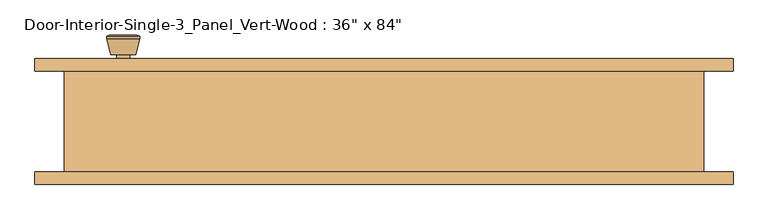
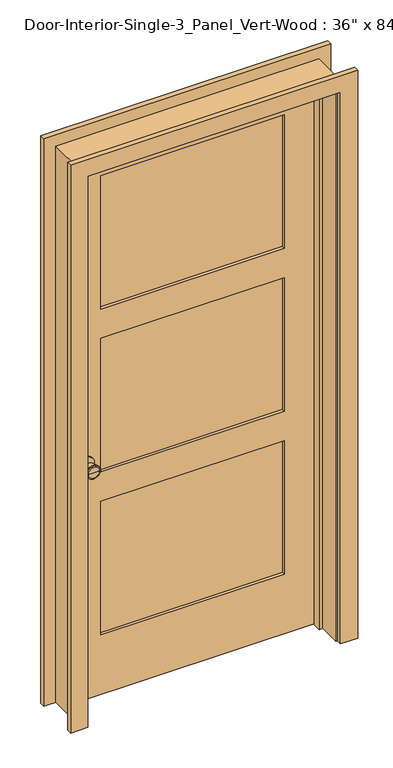
"""IFC4 building model written with IfcOpenShell, lengths in millimetres: door geometry."""

from ifc_helpers import new_model, si_unit, point, frame, frame_2d, origin, place, context, project, spatial, polyline, circle_curve, trimmed, segment, composite_curve, outline, extrude, faceted_brep, source, transform, mapped, element, save
from ifc_brep_helpers import plane_surface, cylinder_surface, revolved_surface, advanced_brep


def door_8959c651(model_context):
    return source(origin(), model_context, "Body", "SolidModel", [
        advanced_brep(
        [(-393.7, 32.1, 914.4), (-383.7, 32.1, 914.4), (-403.7, 32.1, 914.4), (-373.2241324, -16.9, 914.4), (-393.7, -16.9, 914.4), (-414.1758676, -16.9, 914.4), (-368.7, -15.0721319, 914.4), (-418.7, -15.0721319, 914.4), (-368.7, -11.6084537, 914.4), (-418.7, -11.6084537, 914.4), (-375.063764, 13.1, 914.4), (-412.336236, 13.1, 914.4), (-383.7, 13.1, 914.4), (-403.7, 13.1, 914.4)],
        [
            (0, 1),
            (1, 2, circle_curve(frame((-393.7, 32.1, 914.4), z_axis=(0.0, 1.0, 0.0), x_axis=(-1.0, 0.0, 0.0)), 10.0)),
            (2, 0),
            (2, 1, circle_curve(frame((-393.7, 32.1, 914.4), z_axis=(0.0, 1.0, 0.0), x_axis=(-1.0, 0.0, 0.0)), 10.0)),
            (3, 4),
            (4, 5),
            (5, 3, circle_curve(frame((-393.7, -16.9, 914.4), z_axis=(0.0, -1.0, 0.0), x_axis=(-1.0, 0.0, 0.0)), 20.4758676)),
            (3, 5, circle_curve(frame((-393.7, -16.9, 914.4), z_axis=(0.0, -1.0, 0.0), x_axis=(-1.0, 0.0, 0.0)), 20.4758676)),
            (6, 3),
            (5, 7),
            (7, 6, circle_curve(frame((-393.7, -15.0721319, 914.4), z_axis=(0.0, -1.0, 0.0), x_axis=(-1.0, 0.0, 0.0)), 25.0)),
            (6, 7, circle_curve(frame((-393.7, -15.0721319, 914.4), z_axis=(0.0, -1.0, 0.0), x_axis=(-1.0, 0.0, 0.0)), 25.0)),
            (8, 6),
            (7, 9),
            (9, 8, circle_curve(frame((-393.7, -11.6084537, 914.4), z_axis=(0.0, -1.0, 0.0), x_axis=(-1.0, 0.0, 0.0)), 25.0)),
            (8, 9, circle_curve(frame((-393.7, -11.6084537, 914.4), z_axis=(0.0, -1.0, 0.0), x_axis=(-1.0, 0.0, 0.0)), 25.0)),
            (10, 8),
            (9, 11),
            (11, 10, circle_curve(frame((-393.7, 13.1, 914.4), z_axis=(0.0, -1.0, 0.0), x_axis=(-1.0, 0.0, 0.0)), 18.636236)),
            (10, 11, circle_curve(frame((-393.7, 13.1, 914.4), z_axis=(0.0, -1.0, 0.0), x_axis=(-1.0, 0.0, 0.0)), 18.636236)),
            (12, 10),
            (11, 13),
            (13, 12, circle_curve(frame((-393.7, 13.1, 914.4), z_axis=(0.0, -1.0, 0.0), x_axis=(-1.0, 0.0, 0.0)), 10.0)),
            (12, 13, circle_curve(frame((-393.7, 13.1, 914.4), z_axis=(0.0, -1.0, 0.0), x_axis=(-1.0, 0.0, 0.0)), 10.0)),
            (1, 12),
            (13, 2),
        ],
        [
            plane_surface(frame((-393.7, 32.1, 914.4), z_axis=(0.0, 1.0, 0.0), x_axis=(-1.0, 0.0, 0.0))),
            plane_surface(frame((-393.7, -16.9, 914.4), z_axis=(0.0, -1.0, 0.0), x_axis=(-1.0, 0.0, 0.0))),
            revolved_surface(polyline([(-414.1758676, -16.9, 914.4), (-418.7, -15.0721319, 914.4)]), (-393.7, 32.1, 914.4), (0.0, 1.0, 0.0)),
            cylinder_surface(frame((-393.7, 32.1, 914.4), z_axis=(0.0, 1.0, 0.0), x_axis=(-1.0, 0.0, 0.0)), 25.0),
            revolved_surface(polyline([(-418.7, -11.6084537, 914.4), (-412.336236, 13.1, 914.4)]), (-393.7, 32.1, 914.4), (0.0, 1.0, 0.0)),
            plane_surface(frame((-393.7, 13.1, 914.4), z_axis=(0.0, 1.0, 0.0), x_axis=(-1.0, 0.0, 0.0))),
            cylinder_surface(frame((-393.7, 32.1, 914.4), z_axis=(0.0, 1.0, 0.0), x_axis=(-1.0, 0.0, 0.0)), 10.0),
        ],
        [
            (0, [[1, 2, 3]]),
            (0, [[-3, 4, -1]]),
            (1, [[5, 6, 7]]),
            (1, [[-6, -5, 8]]),
            (2, [[9, -7, 10, 11]]),
            (2, [[-10, -8, -9, 12]]),
            (3, [[13, -11, 14, 15]]),
            (3, [[-14, -12, -13, 16]]),
            (4, [[17, -15, 18, 19]]),
            (4, [[-18, -16, -17, 20]]),
            (5, [[21, -19, 22, 23]]),
            (5, [[-22, -20, -21, 24]]),
            (6, [[25, -23, 26, -2]]),
            (6, [[-26, -24, -25, -4]]),
        ],
    ),
        extrude(outline(composite_curve([segment(trimmed(circle_curve(frame_2d((914.4, -393.7)), 30.0), [point((914.4, -423.7))], [point((914.4, -363.7))], False, "CARTESIAN"), True, "CONTINUOUS"), segment(trimmed(circle_curve(frame_2d((914.4, -393.7)), 30.0), [point((914.4, -363.7))], [point((914.4, -423.7))], False, "CARTESIAN"), True, "CONTINUOUS")], self_intersect=False)), frame((0.0, 32.1, 0.0), z_axis=(0.0, 1.0, 0.0), x_axis=(0.0, 0.0, 1.0)), (0.0, 0.0, 1.0), 6.0),
        advanced_brep(
        [(-393.7, 79.025, 914.4), (-403.7, 79.025, 914.4), (-383.7, 79.025, 914.4), (-373.2241324, 128.025, 914.4), (-414.1758676, 128.025, 914.4), (-393.7, 128.025, 914.4), (-368.7, 126.1971319, 914.4), (-418.7, 126.1971319, 914.4), (-368.7, 122.7334537, 914.4), (-418.7, 122.7334537, 914.4), (-375.063764, 98.025, 914.4), (-412.336236, 98.025, 914.4), (-383.7, 98.025, 914.4), (-403.7, 98.025, 914.4)],
        [
            (0, 1),
            (1, 2, circle_curve(frame((-393.7, 79.025, 914.4), z_axis=(0.0, -1.0, 0.0), x_axis=(-1.0, 0.0, 0.0)), 10.0)),
            (2, 0),
            (2, 1, circle_curve(frame((-393.7, 79.025, 914.4), z_axis=(0.0, -1.0, 0.0), x_axis=(-1.0, 0.0, 0.0)), 10.0)),
            (3, 4, circle_curve(frame((-393.7, 128.025, 914.4), z_axis=(0.0, 1.0, 0.0), x_axis=(-1.0, 0.0, 0.0)), 20.4758676)),
            (4, 5),
            (5, 3),
            (4, 3, circle_curve(frame((-393.7, 128.025, 914.4), z_axis=(0.0, 1.0, 0.0), x_axis=(-1.0, 0.0, 0.0)), 20.4758676)),
            (6, 7, circle_curve(frame((-393.7, 126.1971319, 914.4), z_axis=(0.0, 1.0, 0.0), x_axis=(-1.0, 0.0, 0.0)), 25.0)),
            (7, 4),
            (3, 6),
            (7, 6, circle_curve(frame((-393.7, 126.1971319, 914.4), z_axis=(0.0, 1.0, 0.0), x_axis=(-1.0, 0.0, 0.0)), 25.0)),
            (8, 9, circle_curve(frame((-393.7, 122.7334537, 914.4), z_axis=(0.0, 1.0, 0.0), x_axis=(-1.0, 0.0, 0.0)), 25.0)),
            (9, 7),
            (6, 8),
            (9, 8, circle_curve(frame((-393.7, 122.7334537, 914.4), z_axis=(0.0, 1.0, 0.0), x_axis=(-1.0, 0.0, 0.0)), 25.0)),
            (10, 11, circle_curve(frame((-393.7, 98.025, 914.4), z_axis=(0.0, 1.0, 0.0), x_axis=(-1.0, 0.0, 0.0)), 18.636236)),
            (11, 9),
            (8, 10),
            (11, 10, circle_curve(frame((-393.7, 98.025, 914.4), z_axis=(0.0, 1.0, 0.0), x_axis=(-1.0, 0.0, 0.0)), 18.636236)),
            (12, 13, circle_curve(frame((-393.7, 98.025, 914.4), z_axis=(0.0, 1.0, 0.0), x_axis=(-1.0, 0.0, 0.0)), 10.0)),
            (13, 11),
            (10, 12),
            (13, 12, circle_curve(frame((-393.7, 98.025, 914.4), z_axis=(0.0, 1.0, 0.0), x_axis=(-1.0, 0.0, 0.0)), 10.0)),
            (1, 13),
            (12, 2),
        ],
        [
            plane_surface(frame((-393.7, 79.025, 914.4), z_axis=(0.0, -1.0, 0.0), x_axis=(-1.0, 0.0, 0.0))),
            plane_surface(frame((-393.7, 128.025, 914.4), z_axis=(0.0, 1.0, 0.0), x_axis=(-1.0, 0.0, 0.0))),
            revolved_surface(polyline([(-414.1758676, 128.025, 914.4), (-418.7, 126.1971319, 914.4)]), (-393.7, 79.025, 914.4), (0.0, -1.0, 0.0)),
            cylinder_surface(frame((-393.7, 79.025, 914.4), z_axis=(0.0, -1.0, 0.0), x_axis=(-1.0, 0.0, 0.0)), 25.0),
            revolved_surface(polyline([(-418.7, 122.7334537, 914.4), (-412.336236, 98.025, 914.4)]), (-393.7, 79.025, 914.4), (0.0, -1.0, 0.0)),
            plane_surface(frame((-393.7, 98.025, 914.4), z_axis=(0.0, -1.0, 0.0), x_axis=(-1.0, 0.0, 0.0))),
            cylinder_surface(frame((-393.7, 79.025, 914.4), z_axis=(0.0, -1.0, 0.0), x_axis=(-1.0, 0.0, 0.0)), 10.0),
        ],
        [
            (0, [[1, 2, 3]]),
            (0, [[-3, 4, -1]]),
            (1, [[5, 6, 7]]),
            (1, [[8, -7, -6]]),
            (2, [[9, 10, -5, 11]]),
            (2, [[12, -11, -8, -10]]),
            (3, [[13, 14, -9, 15]]),
            (3, [[16, -15, -12, -14]]),
            (4, [[17, 18, -13, 19]]),
            (4, [[20, -19, -16, -18]]),
            (5, [[21, 22, -17, 23]]),
            (5, [[24, -23, -20, -22]]),
            (6, [[-2, 25, -21, 26]]),
            (6, [[-4, -26, -24, -25]]),
        ],
    ),
        extrude(outline(composite_curve([segment(trimmed(circle_curve(frame_2d((914.4, -393.7)), 30.0), [point((914.4, -423.7))], [point((914.4, -363.7))], False, "CARTESIAN"), True, "CONTINUOUS"), segment(trimmed(circle_curve(frame_2d((914.4, -393.7)), 30.0), [point((914.4, -363.7))], [point((914.4, -423.7))], False, "CARTESIAN"), True, "CONTINUOUS")], self_intersect=False)), frame((0.0, 73.025, 0.0), z_axis=(0.0, 1.0, 0.0), x_axis=(0.0, 0.0, 1.0)), (0.0, 0.0, 1.0), 6.0),
        extrude(outline(polyline([(336.55, 49.7416667), (-336.55, 49.7416667), (-336.55, 61.3833333), (336.55, 61.3833333), (336.55, 49.7416667)])), frame((0.0, 0.0, 1496.4833333), z_axis=(0.0, 0.0, 1.0), x_axis=(1.0, 0.0, 0.0)), (0.0, 0.0, 1.0), 518.0541667),
        extrude(outline(polyline([(336.55, 49.7416667), (-336.55, 49.7416667), (-336.55, 61.3833333), (336.55, 61.3833333), (336.55, 49.7416667)])), frame((0.0, 0.0, 231.775), z_axis=(0.0, 0.0, 1.0), x_axis=(1.0, 0.0, 0.0)), (0.0, 0.0, 1.0), 518.0541667),
        extrude(outline(polyline([(336.55, 49.7416667), (-336.55, 49.7416667), (-336.55, 61.3833333), (336.55, 61.3833333), (336.55, 49.7416667)])), frame((0.0, 0.0, 864.1291667), z_axis=(0.0, 0.0, 1.0), x_axis=(1.0, 0.0, 0.0)), (0.0, 0.0, 1.0), 518.0541667),
        extrude(outline(polyline([(2133.6, -457.2), (0.0, -457.2), (0.0, 457.2), (2133.6, 457.2), (2133.6, -457.2)]), holes=[polyline([(2014.5375, -336.55), (2014.5375, 336.55), (1496.4833333, 336.55), (1496.4833333, -336.55), (2014.5375, -336.55)]), polyline([(749.8291667, -336.55), (749.8291667, 336.55), (231.775, 336.55), (231.775, -336.55), (749.8291667, -336.55)]), polyline([(1382.1833333, -336.55), (1382.1833333, 336.55), (864.1291667, 336.55), (864.1291667, -336.55), (1382.1833333, -336.55)])]), frame((0.0, 38.1, 0.0), z_axis=(0.0, 1.0, 0.0), x_axis=(0.0, 0.0, 1.0)), (0.0, 0.0, 1.0), 34.925),
        faceted_brep([(482.6, 73.025, 0.0), (482.6, -79.375, 0.0), (457.2, -79.375, 0.0), (457.2, 3.175, 0.0), (444.5, 3.175, 0.0), (444.5, 38.1, 0.0), (457.2, 38.1, 0.0), (457.2, 73.025, 0.0), (482.6, 73.025, 2159.0), (482.6, -79.375, 2159.0), (-482.6, -79.375, 2159.0), (-482.6, -79.375, 0.0), (-457.2, -79.375, 0.0), (-457.2, -79.375, 2133.6), (457.2, -79.375, 2133.6), (457.2, 3.175, 2133.6), (-457.2, 3.175, 2133.6), (-457.2, 3.175, 0.0), (-444.5, 3.175, 0.0), (-444.5, 3.175, 2120.9), (444.5, 3.175, 2120.9), (444.5, 38.1, 2120.9), (-444.5, 38.1, 2120.9), (-444.5, 38.1, 0.0), (-457.2, 38.1, 0.0), (-457.2, 38.1, 2133.6), (457.2, 38.1, 2133.6), (457.2, 73.025, 2133.6), (-457.2, 73.025, 2133.6), (-457.2, 73.025, 0.0), (-482.6, 73.025, 0.0), (-482.6, 73.025, 2159.0)], [[[0, 1, 2, 3, 4, 5, 6, 7]], [[1, 0, 8, 9]], [[2, 1, 9, 10, 11, 12, 13, 14]], [[3, 2, 14, 15]], [[4, 3, 15, 16, 17, 18, 19, 20]], [[5, 4, 20, 21]], [[6, 5, 21, 22, 23, 24, 25, 26]], [[7, 6, 26, 27]], [[0, 7, 27, 28, 29, 30, 31, 8]], [[9, 8, 31, 10]], [[15, 14, 13, 16]], [[21, 20, 19, 22]], [[27, 26, 25, 28]], [[30, 29, 24, 23, 18, 17, 12, 11]], [[10, 31, 30, 11]], [[16, 13, 12, 17]], [[22, 19, 18, 23]], [[28, 25, 24, 29]]]),
        extrude(outline(polyline([(0.0, 463.55), (0.0, 527.05), (2203.45, 527.05), (2203.45, -527.05), (0.0, -527.05), (0.0, -463.55), (2139.95, -463.55), (2139.95, 463.55), (0.0, 463.55)])), frame((0.0, -98.425, 0.0), z_axis=(0.0, 1.0, 0.0), x_axis=(0.0, 0.0, 1.0)), (0.0, 0.0, 1.0), 19.05),
        extrude(outline(polyline([(0.0, 463.55), (0.0, 527.05), (2203.45, 527.05), (2203.45, -527.05), (0.0, -527.05), (0.0, -463.55), (2139.95, -463.55), (2139.95, 463.55), (0.0, 463.55)])), frame((0.0, 73.025, 0.0), z_axis=(0.0, 1.0, 0.0), x_axis=(0.0, 0.0, 1.0)), (0.0, 0.0, 1.0), 19.05),
    ])


if __name__ == "__main__":
    model = new_model("IFC4")
    model_context = context("Model", 3, world=origin())
    ifc_project = project(units=[si_unit("LENGTHUNIT", "METRE", prefix="MILLI")], contexts=[model_context])
    site = spatial("IfcSite", under=ifc_project)
    building = spatial("IfcBuilding", under=site)
    placement = place(None, origin())
    door_shape = door_8959c651(model_context)
    element("IfcDoor", 1, ObjectType="Door-Interior-Single-3_Panel_Vert-Wood : 36\" x 84\"", at=placement, inside=building, context=model_context, shape_type="MappedRepresentation", body=[
        mapped(door_shape, transform((0.0, 0.0, 0.0), x_axis=(1.0, 0.0, 0.0), y_axis=(0.0, 1.0, 0.0), z_axis=(0.0, 0.0, 1.0))),
    ])
    save(model, "model.ifc")

# Revit data of these elements
# Type "Door-Interior-Single-3_Panel_Vert-Wood : 36\" x 84\""
#   Type Mark = "9"
#   Assembly Code = "C1020300"
#   Analytic Construction = "Wooden"
#   Top Rail = 0' - 4 11/16"
#   Thickness = 0' - 1 3/8"
#   Thermal Resistance (R) = 2.5876 (h·ft²·°F)/BTU
#   Swing Angle [instance default] = 90.00°
#   Stiles = 0' - 4 3/4"
#   Rough Width = 3' - 2"
#   Rough Height = 7' - 1"
#   Intermediate Rail = 0' - 4 1/2"
#   Height = 7' - 0"
#   Width = 3' - 0"
#   Heat Transfer Coefficient (U) = 0.3865 BTU/(h·ft²·°F)
#   Bottom Rail = 0' - 9 1/8"
#   Trim Material = Cherry
#   Panel Material = Cherry
#   Frame Material = Cherry
#   Door Handle Material = Aluminum
#   Visual Light Transmittance = 0
#   Solar Heat Gain Coefficient = 0
#   Wall Closure = (empty or 0)
#   Function = (empty or 0)
# Element 1 (IfcDoor, "Door-Interior-Single-3_Panel_Vert-Wood : 36\" x 84\"")
#   Materials on its faces: "Cherry", "Aluminum"
# Materials
#   "Cherry": class "Wood", colour RGB 226 177 128, transparency 0, Description = "Prunus Serotina", Cost = 0
#   "Aluminum": class "Metal", colour RGB 247 247 247, transparency 0, Description = "Aluminum 6061", Cost = 0
